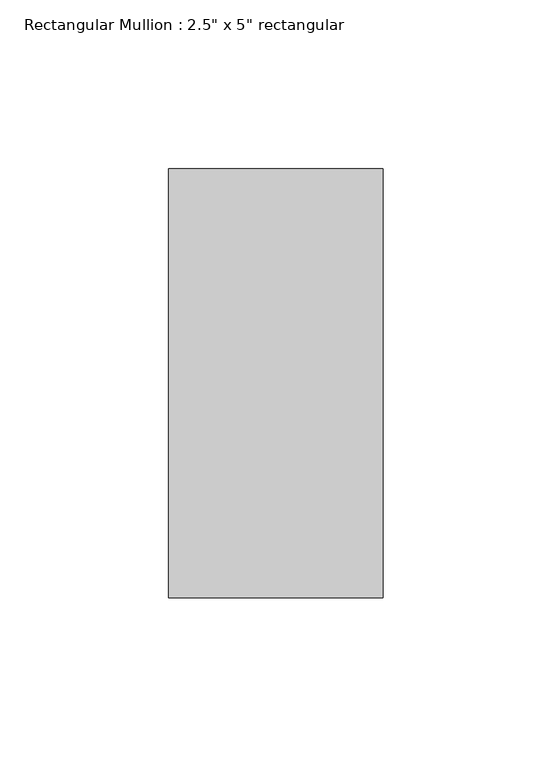
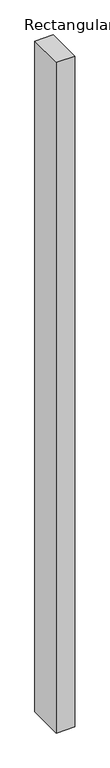
"""IFC4 building model written with IfcOpenShell, lengths in millimetres: member geometry."""

from ifc_helpers import new_model, si_unit, frame, origin, place, context, project, spatial, polyline, outline, extrude, source, transform, mapped, element, save


def member_ee409385(model_context):
    return source(origin(), model_context, "Body", "SweptSolid", [
        extrude(outline(polyline([(0.0, 63.5), (0.0, -63.5), (-63.5, -63.5), (-63.5, 63.5), (0.0, 63.5)])), frame((0.0, 0.0, -2438.4), z_axis=(0.0, 0.0, 1.0), x_axis=(1.0, 0.0, 0.0)), (0.0, 0.0, 1.0), 2438.4),
    ])


if __name__ == "__main__":
    model = new_model("IFC4")
    model_context = context("Model", 3, world=origin())
    ifc_project = project(units=[si_unit("LENGTHUNIT", "METRE", prefix="MILLI")], contexts=[model_context])
    site = spatial("IfcSite", under=ifc_project)
    building = spatial("IfcBuilding", under=site)
    placement = place(None, origin())
    member_shape = member_ee409385(model_context)
    element("IfcMember", 1, ObjectType="Rectangular Mullion : 2.5\" x 5\" rectangular", at=placement, inside=building, context=model_context, shape_type="MappedRepresentation", body=[
        mapped(member_shape, transform((0.0, 0.0, 0.0), x_axis=(1.0, 0.0, 0.0), y_axis=(0.0, 1.0, 0.0), z_axis=(0.0, 0.0, 1.0))),
    ])
    save(model, "model.ifc")

# Revit data of these elements
# Type "Rectangular Mullion : 2.5\" x 5\" rectangular"
#   built-in parameter 1007304 = 0.416667 (stored number, unit not read)
#   built-in parameter 1007301 = 0.104167 (stored number, unit not read)
#   built-in parameter 1007300 = 0.104167 (stored number, unit not read)
# Element 1 (IfcMember, "Rectangular Mullion : 2.5\" x 5\" rectangular")
#   Materials on its faces: "Iron, Ductile"
# Materials
#   "Iron, Ductile": class "Metal", colour RGB 0 0 0, transparency 0, Description = "Ductile cast iron", Cost = 0
